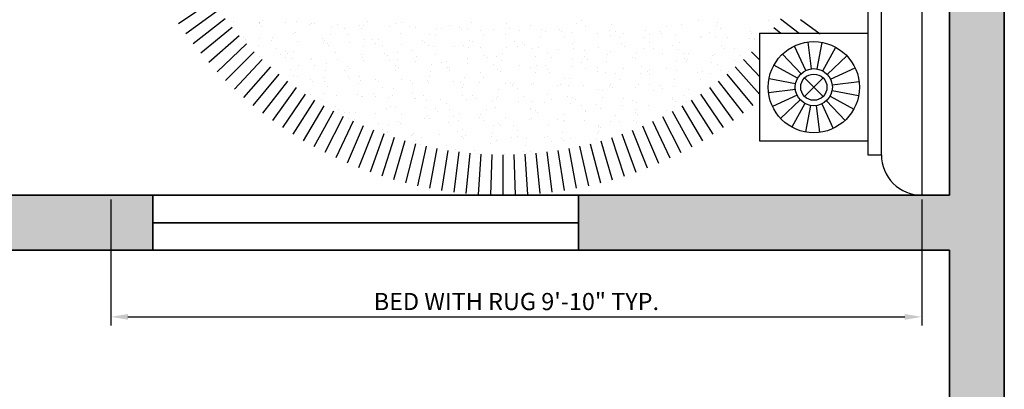
# Model space of a CAD drawing. Units: inches. Extents: x 1566 to 2546, y 1087 to 2705.
# Tile 15 of 27: x 2315 to 2458, y 1189 to 1243. Entities that reach past the tile are written whole.
import ezdxf

# ---------------------------------------------------------------- set-up
doc = ezdxf.new("R2010")
doc.units = ezdxf.units.IN
for name, color, linetype, lineweight in [('A-ANNO-DIMS', 2, 'Continuous', 18), ('A-FURN', 8, 'Continuous', 18), ('A-WALL', 7, 'Continuous', 35), ('A-WALL-PATT', 8, 'Continuous', 13)]:
    doc.layers.add(name, color=color, linetype=linetype, lineweight=lineweight)
for name, color, linetype in [('A-FRN', 11, 'Continuous'), ('A-HT', 15, 'Continuous'), ('L-HT', 1, 'Continuous')]:
    doc.layers.add(name, color=color, linetype=linetype)
doc.styles.get("Standard").update_dxf_attribs({"font": 'arial.ttf'})
doc.dimstyles.new('ISO-25', dxfattribs={"dimtxt": 2.5, "dimasz": 2.5, "dimexe": 1.25, "dimexo": 0.625, "dimtad": 1, "dimtxsty": 'Standard', "dimcen": 2.5, "dimadec": 0, "dimazin": 0, "dimtfac": 1, "dimtmove": 0, "dimatfit": 3, "dimfxl": 1, "dimarcsym": 0})

# ---------------------------------------------------------------- blocks, each defined once
blk = doc.blocks.new('*X21')
at = {"color": 0}
for p, q in [((2.8058, 2.548), (2.8058, 2.548)), ((2.8678, 2.5109), (2.8678, 2.5109)), ((2.8734, 2.5011), (2.8734, 2.5011)), ((2.8889, 2.4975), (2.8889, 2.4975)), ((2.8024, 2.4403), (2.8024, 2.4403)), ((2.8089, 2.4516), (2.8089, 2.4516)), ((2.8091, 2.4488), (2.8091, 2.4488)), ((2.8148, 2.4495), (2.8148, 2.4495)), ((2.824, 2.4411), (2.824, 2.4411)), ((2.8703, 2.4492), (2.8703, 2.4492)), ((2.8963, 2.4526), (2.8963, 2.4526)), ((2.9368, 2.451), (2.9368, 2.451)), ((2.8765, 2.4048), (2.8765, 2.4048)), ((2.8675, 2.4012), (2.8675, 2.4012)), ((2.9082, 2.3857), (2.9082, 2.3857)), ((2.9293, 2.3723), (2.9293, 2.3723)), ((2.8121, 2.3553), (2.8121, 2.3553)), ((2.9173, 2.3556), (2.9173, 2.3556)), ((2.9265, 2.3472), (2.9265, 2.3472)), ((2.94, 2.3547), (2.94, 2.3547)), ((2.983, 2.3346), (2.983, 2.3346)), ((2.8078, 2.3115), (2.8078, 2.3115)), ((2.8485, 2.3169), (2.8485, 2.3169)), ((2.8495, 2.3236), (2.8495, 2.3236)), ((2.8797, 2.3084), (2.8797, 2.3084)), ((2.9164, 2.3258), (2.9164, 2.3258)), ((2.9424, 2.3292), (2.9424, 2.3292)), ((2.97, 2.3073), (2.97, 2.3073)), ((3.0052, 2.3239), (3.0052, 2.3239)), ((3.0106, 2.3101), (3.0106, 2.3101)), ((2.8152, 2.259), (2.8152, 2.259)), ((2.8197, 2.2634), (2.8197, 2.2634)), ((2.9431, 2.2584), (2.9431, 2.2584)), ((2.9486, 2.2605), (2.9486, 2.2605)), ((3.0198, 2.2617), (3.0198, 2.2617)), ((3.0782, 2.2632), (3.0782, 2.2632)), ((2.814, 2.2468), (2.814, 2.2468)), ((2.9697, 2.2471), (2.9697, 2.2471)), ((3.029, 2.2533), (3.029, 2.2533)), ((2.8539, 2.1881), (2.8539, 2.1881)), ((2.8695, 2.2178), (2.8695, 2.2178)), ((2.8787, 2.2094), (2.8787, 2.2094)), ((2.8828, 2.2121), (2.8828, 2.2121)), ((2.8899, 2.1984), (2.8899, 2.1984)), ((2.8946, 2.1935), (2.8946, 2.1935)), ((2.9625, 2.2024), (2.9625, 2.2024)), ((2.9885, 2.2058), (2.9885, 2.2058)), ((3.0137, 2.2138), (3.0137, 2.2138)), ((3.0291, 2.2112), (3.0291, 2.2112)), ((3.0456, 2.1987), (3.0456, 2.1987)), ((3.0725, 2.2134), (3.0725, 2.2134)), ((3.0971, 2.2201), (3.0971, 2.2201)), ((2.8184, 2.1626), (2.8184, 2.1626)), ((2.8279, 2.1847), (2.8279, 2.1847)), ((2.9222, 2.1695), (2.9222, 2.1695)), ((2.9463, 2.162), (2.9463, 2.162)), ((3.0813, 2.1669), (3.0813, 2.1669)), ((3.1223, 2.1678), (3.1223, 2.1678)), ((3.1315, 2.1594), (3.1315, 2.1594)), ((2.8333, 2.135), (2.8333, 2.135)), ((2.8544, 2.1216), (2.8544, 2.1216)), ((2.886, 2.1157), (2.886, 2.1157)), ((2.972, 2.1239), (2.972, 2.1239)), ((2.9812, 2.1155), (2.9812, 2.1155)), ((2.989, 2.1353), (2.989, 2.1353)), ((3.0101, 2.1218), (3.0101, 2.1218)), ((3.0169, 2.1174), (3.0169, 2.1174)), ((3.1447, 2.1356), (3.1447, 2.1356)), ((3.1448, 2.1168), (3.1448, 2.1168)), ((3.1658, 2.1221), (3.1658, 2.1221)), ((2.8216, 2.08), (2.8216, 2.08)), ((3.0086, 2.079), (3.0086, 2.079)), ((3.0346, 2.0825), (3.0346, 2.0825)), ((3.0752, 2.0878), (3.0752, 2.0878)), ((3.1432, 2.0968), (3.1432, 2.0968)), ((3.1692, 2.1002), (3.1692, 2.1002)), ((2.8061, 2.0524), (2.8061, 2.0524)), ((2.8215, 2.0663), (2.8215, 2.0663)), ((2.8309, 2.0716), (2.8309, 2.0716)), ((2.874, 2.0613), (2.874, 2.0613)), ((2.9, 2.0647), (2.9, 2.0647)), ((2.9303, 2.0732), (2.9303, 2.0732)), ((2.9407, 2.0701), (2.9407, 2.0701)), ((2.9494, 2.0657), (2.9494, 2.0657)), ((3.0247, 2.0756), (3.0247, 2.0756)), ((3.0845, 2.0705), (3.0845, 2.0705)), ((3.086, 2.0735), (3.086, 2.0735)), ((2.8737, 2.0098), (2.8737, 2.0098)), ((2.8744, 2.0317), (2.8744, 2.0317)), ((2.8891, 2.0194), (2.8891, 2.0194)), ((3.02, 2.0211), (3.02, 2.0211)), ((3.0294, 2.0101), (3.0294, 2.0101)), ((3.0744, 2.03), (3.0744, 2.03)), ((3.0837, 2.0216), (3.0837, 2.0216)), ((3.1479, 2.0205), (3.1479, 2.0205)), ((3.1851, 2.0104), (3.1851, 2.0104)), ((2.8247, 1.9699), (2.8247, 1.9699)), ((2.8947, 1.9964), (2.8947, 1.9964)), ((2.9241, 1.9861), (2.9241, 1.9861)), ((2.9333, 1.9777), (2.9333, 1.9777)), ((2.9526, 1.9693), (2.9526, 1.9693)), ((3.0505, 1.9966), (3.0505, 1.9966)), ((3.0876, 1.9742), (3.0876, 1.9742)), ((3.1272, 1.9817), (3.1272, 1.9817)), ((3.1893, 1.9734), (3.1893, 1.9734)), ((3.2062, 1.9969), (3.2062, 1.9969)), ((3.2153, 1.9768), (3.2153, 1.9768)), ((3.2185, 1.9759), (3.2185, 1.9759)), ((2.8149, 1.9477), (2.8149, 1.9477)), ((2.9201, 1.9379), (2.9201, 1.9379)), ((2.9461, 1.9414), (2.9461, 1.9414)), ((2.9707, 1.948), (2.9707, 1.948)), ((2.9768, 1.9378), (2.9768, 1.9378)), ((2.9868, 1.9467), (2.9868, 1.9467)), ((3.0547, 1.9556), (3.0547, 1.9556)), ((3.0807, 1.9591), (3.0807, 1.9591)), ((3.1213, 1.9644), (3.1213, 1.9644)), ((3.1264, 1.9483), (3.1264, 1.9483)), ((3.1769, 1.9361), (3.1769, 1.9361)), ((2.8115, 1.9236), (2.8115, 1.9236)), ((2.8265, 1.894), (2.8265, 1.894)), ((2.8522, 1.929), (2.8522, 1.929)), ((2.8923, 1.9231), (2.8923, 1.9231)), ((3.0232, 1.9247), (3.0232, 1.9247)), ((3.1511, 1.9241), (3.1511, 1.9241)), ((3.1861, 1.9277), (3.1861, 1.9277)), ((2.8278, 1.8736), (2.8278, 1.8736)), ((2.914, 1.8846), (2.914, 1.8846)), ((2.9351, 1.8712), (2.9351, 1.8712)), ((2.9557, 1.873), (2.9557, 1.873)), ((3.0266, 1.8922), (3.0266, 1.8922)), ((3.0358, 1.8838), (3.0358, 1.8838)), ((3.0697, 1.8849), (3.0697, 1.8849)), ((3.0908, 1.8779), (3.0908, 1.8779)), ((3.0908, 1.8714), (3.0908, 1.8714)), ((3.2217, 1.8795), (3.2217, 1.8795)), ((3.2255, 1.8852), (3.2255, 1.8852)), ((3.2296, 1.8878), (3.2296, 1.8878)), ((3.2465, 1.8717), (3.2465, 1.8717)), ((2.8553, 1.8225), (2.8553, 1.8225)), ((2.8763, 1.8484), (2.8763, 1.8484)), ((2.8855, 1.8399), (2.8855, 1.8399)), ((2.8954, 1.8267), (2.8954, 1.8267)), ((3.011, 1.8228), (3.011, 1.8228)), ((3.0263, 1.8284), (3.0263, 1.8284)), ((3.0329, 1.8233), (3.0329, 1.8233)), ((3.0793, 1.8439), (3.0793, 1.8439)), ((3.1008, 1.8323), (3.1008, 1.8323)), ((3.1268, 1.8357), (3.1268, 1.8357)), ((3.1542, 1.8278), (3.1542, 1.8278)), ((3.1667, 1.8231), (3.1667, 1.8231)), ((3.1674, 1.841), (3.1674, 1.841)), ((3.2354, 1.85), (3.2354, 1.85)), ((3.2614, 1.8534), (3.2614, 1.8534)), ((2.8316, 1.7968), (2.8316, 1.7968)), ((2.8576, 1.8002), (2.8576, 1.8002)), ((2.8983, 1.8056), (2.8983, 1.8056)), ((2.929, 1.8), (2.929, 1.8)), ((2.9662, 1.8145), (2.9662, 1.8145)), ((2.9922, 1.818), (2.9922, 1.818)), ((3.1291, 1.7983), (3.1291, 1.7983)), ((3.1383, 1.7899), (3.1383, 1.7899)), ((2.831, 1.7773), (2.831, 1.7773)), ((2.9544, 1.7594), (2.9544, 1.7594)), ((2.9589, 1.7766), (2.9589, 1.7766)), ((2.9788, 1.7544), (2.9788, 1.7544)), ((3.0939, 1.7815), (3.0939, 1.7815)), ((3.1101, 1.7597), (3.1101, 1.7597)), ((3.1818, 1.75), (3.1818, 1.75)), ((3.2248, 1.7832), (3.2248, 1.7832)), ((3.2658, 1.7599), (3.2658, 1.7599)), ((2.8198, 1.7457), (2.8198, 1.7457)), ((2.8986, 1.7304), (2.8986, 1.7304)), ((2.9755, 1.7459), (2.9755, 1.7459)), ((2.988, 1.746), (2.988, 1.746)), ((3.0295, 1.7321), (3.0295, 1.7321)), ((3.1312, 1.7462), (3.1312, 1.7462)), ((3.1574, 1.7314), (3.1574, 1.7314)), ((3.1729, 1.7123), (3.1729, 1.7123)), ((3.2135, 1.7176), (3.2135, 1.7176)), ((3.2815, 1.7266), (3.2815, 1.7266)), ((2.8285, 1.7106), (2.8285, 1.7106)), ((2.8341, 1.6809), (2.8341, 1.6809)), ((2.8377, 1.7021), (2.8377, 1.7021)), ((2.8957, 1.6973), (2.8957, 1.6973)), ((2.9037, 1.6769), (2.9037, 1.6769)), ((2.9444, 1.6822), (2.9444, 1.6822)), ((2.962, 1.6803), (2.962, 1.6803)), ((3.0123, 1.6911), (3.0123, 1.6911)), ((3.0315, 1.7061), (3.0315, 1.7061)), ((3.0383, 1.6946), (3.0383, 1.6946)), ((3.0514, 1.6976), (3.0514, 1.6976)), ((3.079, 1.6999), (3.079, 1.6999)), ((3.0971, 1.6852), (3.0971, 1.6852)), ((3.1469, 1.7089), (3.1469, 1.7089)), ((3.2071, 1.6979), (3.2071, 1.6979)), ((3.228, 1.6868), (3.228, 1.6868)), ((3.2316, 1.7044), (3.2316, 1.7044)), ((3.2408, 1.696), (3.2408, 1.696)), ((2.8098, 1.6645), (2.8098, 1.6645)), ((2.8777, 1.6734), (2.8777, 1.6734)), ((2.8812, 1.6623), (2.8812, 1.6623)), ((3.0813, 1.6605), (3.0813, 1.6605)), ((3.0905, 1.6521), (3.0905, 1.6521)), ((3.2843, 1.6561), (3.2843, 1.6561)), ((3.2956, 1.64), (3.2956, 1.64)), ((2.8391, 1.6339), (2.8391, 1.6339)), ((2.8602, 1.6205), (2.8602, 1.6205)), ((2.9017, 1.634), (2.9017, 1.634)), ((2.931, 1.6167), (2.931, 1.6167)), ((2.9402, 1.6082), (2.9402, 1.6082)), ((2.9948, 1.6342), (2.9948, 1.6342)), ((3.0159, 1.6207), (3.0159, 1.6207)), ((3.0326, 1.6357), (3.0326, 1.6357)), ((3.134, 1.6122), (3.134, 1.6122)), ((3.1505, 1.6345), (3.1505, 1.6345)), ((3.1605, 1.6351), (3.1605, 1.6351)), ((3.1716, 1.621), (3.1716, 1.621)), ((2.8373, 1.5846), (2.8373, 1.5846)), ((2.9361, 1.5721), (2.9361, 1.5721)), ((2.9652, 1.584), (2.9652, 1.584)), ((2.9837, 1.5683), (2.9837, 1.5683)), ((3.0584, 1.5678), (3.0584, 1.5678)), ((3.0844, 1.5712), (3.0844, 1.5712)), ((3.0918, 1.5724), (3.0918, 1.5724)), ((3.1002, 1.5888), (3.1002, 1.5888)), ((3.1251, 1.5765), (3.1251, 1.5765)), ((3.1838, 1.5666), (3.1838, 1.5666)), ((3.193, 1.5855), (3.193, 1.5855)), ((3.219, 1.5889), (3.219, 1.5889)), ((3.2311, 1.5905), (3.2311, 1.5905)), ((3.2475, 1.5727), (3.2475, 1.5727)), ((3.2596, 1.5943), (3.2596, 1.5943)), ((2.8152, 1.5357), (2.8152, 1.5357)), ((2.8559, 1.5411), (2.8559, 1.5411)), ((2.9049, 1.5377), (2.9049, 1.5377)), ((2.9238, 1.55), (2.9238, 1.55)), ((2.9498, 1.5535), (2.9498, 1.5535)), ((2.9905, 1.5588), (2.9905, 1.5588)), ((3.0358, 1.5394), (3.0358, 1.5394)), ((3.1637, 1.5388), (3.1637, 1.5388)), ((3.193, 1.5582), (3.193, 1.5582)), ((3.2987, 1.5436), (3.2987, 1.5436)), ((2.8334, 1.5245), (2.8334, 1.5245)), ((2.8795, 1.5087), (2.8795, 1.5087)), ((2.9006, 1.4953), (2.9006, 1.4953)), ((3.0334, 1.5227), (3.0334, 1.5227)), ((3.0352, 1.509), (3.0352, 1.509)), ((3.0427, 1.5143), (3.0427, 1.5143)), ((3.0563, 1.4955), (3.0563, 1.4955)), ((3.1909, 1.5093), (3.1909, 1.5093)), ((3.212, 1.4958), (3.212, 1.4958)), ((3.2343, 1.4942), (3.2343, 1.4942)), ((3.2365, 1.5183), (3.2365, 1.5183)), ((2.8404, 1.4882), (2.8404, 1.4882)), ((2.8831, 1.4789), (2.8831, 1.4789)), ((2.8924, 1.4704), (2.8924, 1.4704)), ((2.9683, 1.4876), (2.9683, 1.4876)), ((3.0862, 1.4744), (3.0862, 1.4744)), ((3.1034, 1.4925), (3.1034, 1.4925)), ((3.2391, 1.4621), (3.2391, 1.4621)), ((3.2651, 1.4655), (3.2651, 1.4655)), ((3.2862, 1.4727), (3.2862, 1.4727)), ((3.2954, 1.4643), (3.2954, 1.4643)), ((2.8208, 1.4466), (2.8208, 1.4466)), ((2.908, 1.4414), (2.908, 1.4414)), ((2.9359, 1.4306), (2.9359, 1.4306)), ((2.9699, 1.4267), (2.9699, 1.4267)), ((2.9765, 1.4469), (2.9765, 1.4469)), ((2.9959, 1.4301), (2.9959, 1.4301)), ((3.0366, 1.4354), (3.0366, 1.4354)), ((3.0389, 1.443), (3.0389, 1.443)), ((3.1045, 1.4444), (3.1045, 1.4444)), ((3.1305, 1.4478), (3.1305, 1.4478)), ((3.1322, 1.4472), (3.1322, 1.4472)), ((3.1359, 1.4288), (3.1359, 1.4288)), ((3.1451, 1.4204), (3.1451, 1.4204)), ((3.1668, 1.4424), (3.1668, 1.4424)), ((3.1712, 1.4532), (3.1712, 1.4532)), ((3.2879, 1.4475), (3.2879, 1.4475)), ((2.8353, 1.4089), (2.8353, 1.4089)), ((2.8436, 1.3919), (2.8436, 1.3919)), ((2.8613, 1.4124), (2.8613, 1.4124)), ((2.902, 1.4177), (2.902, 1.4177)), ((2.9715, 1.3913), (2.9715, 1.3913)), ((2.9856, 1.385), (2.9856, 1.385)), ((3.0756, 1.3838), (3.0756, 1.3838)), ((3.1065, 1.3961), (3.1065, 1.3961)), ((3.2313, 1.384), (3.2313, 1.384)), ((3.2374, 1.3978), (3.2374, 1.3978)), ((2.9199, 1.3835), (2.9199, 1.3835)), ((2.9409, 1.37), (2.9409, 1.37)), ((2.9948, 1.3765), (2.9948, 1.3765)), ((3.0967, 1.3703), (3.0967, 1.3703)), ((3.1886, 1.3805), (3.1886, 1.3805)), ((3.2524, 1.3706), (3.2524, 1.3706)), ((2.8353, 1.3411), (2.8353, 1.3411)), ((2.8445, 1.3326), (2.8445, 1.3326)), ((2.8611, 1.3214), (2.8611, 1.3214)), ((2.9112, 1.345), (2.9112, 1.345)), ((3.0169, 1.3217), (3.0169, 1.3217)), ((3.0383, 1.3367), (3.0383, 1.3367)), ((3.0421, 1.3467), (3.0421, 1.3467)), ((3.0827, 1.312), (3.0827, 1.312)), ((3.1506, 1.321), (3.1506, 1.321)), ((3.17, 1.3461), (3.17, 1.3461)), ((3.1726, 1.322), (3.1726, 1.322)), ((3.1766, 1.3244), (3.1766, 1.3244)), ((3.2173, 1.3298), (3.2173, 1.3298)), ((3.2384, 1.3349), (3.2384, 1.3349)), ((3.2476, 1.3265), (3.2476, 1.3265)), ((2.8135, 1.2766), (2.8135, 1.2766)), ((2.8467, 1.2956), (2.8467, 1.2956)), ((2.8814, 1.2855), (2.8814, 1.2855)), ((2.888, 1.2928), (2.888, 1.2928)), ((2.9074, 1.289), (2.9074, 1.289)), ((2.9481, 1.2943), (2.9481, 1.2943)), ((2.9746, 1.2949), (2.9746, 1.2949)), ((3.016, 1.3033), (3.016, 1.3033)), ((3.042, 1.3067), (3.042, 1.3067)), ((3.0881, 1.291), (3.0881, 1.291)), ((3.0973, 1.2826), (3.0973, 1.2826)), ((3.1097, 1.2998), (3.1097, 1.2998)), ((3.2406, 1.3015), (3.2406, 1.3015)), ((2.8045, 1.258), (2.8045, 1.258)), ((2.8256, 1.2446), (2.8256, 1.2446)), ((2.9143, 1.2487), (2.9143, 1.2487)), ((2.9378, 1.2472), (2.9378, 1.2472)), ((2.947, 1.2387), (2.947, 1.2387)), ((2.9602, 1.2583), (2.9602, 1.2583)), ((2.9813, 1.2448), (2.9813, 1.2448)), ((3.0452, 1.2503), (3.0452, 1.2503)), ((3.1159, 1.2586), (3.1159, 1.2586)), ((3.137, 1.2451), (3.137, 1.2451)), ((3.1408, 1.2427), (3.1408, 1.2427)), ((3.1731, 1.2497), (3.1731, 1.2497)), ((3.1128, 1.2035), (3.1128, 1.2035)), ((3.2437, 1.2051), (3.2437, 1.2051)), ((2.8499, 1.1992), (2.8499, 1.1992)), ((2.9015, 1.1962), (2.9015, 1.1962)), ((2.9535, 1.1656), (2.9535, 1.1656)), ((2.9778, 1.1986), (2.9778, 1.1986)), ((2.9905, 1.1989), (2.9905, 1.1989)), ((2.9942, 1.1709), (2.9942, 1.1709)), ((3.0572, 1.1965), (3.0572, 1.1965)), ((3.0621, 1.1799), (3.0621, 1.1799)), ((3.0881, 1.1833), (3.0881, 1.1833)), ((3.1288, 1.1887), (3.1288, 1.1887)), ((3.1906, 1.1971), (3.1906, 1.1971)), ((3.1967, 1.1976), (3.1967, 1.1976)), ((3.1998, 1.1887), (3.1998, 1.1887)), ((3.2129, 1.1968), (3.2129, 1.1968)), ((3.2227, 1.201), (3.2227, 1.201)), ((2.8189, 1.1479), (2.8189, 1.1479)), ((2.8402, 1.155), (2.8402, 1.155)), ((2.8449, 1.1328), (2.8449, 1.1328)), ((2.8596, 1.1532), (2.8596, 1.1532)), ((2.9175, 1.1523), (2.9175, 1.1523)), ((2.9275, 1.1622), (2.9275, 1.1622)), ((3.0006, 1.1331), (3.0006, 1.1331)), ((3.0403, 1.1533), (3.0403, 1.1533)), ((3.0484, 1.154), (3.0484, 1.154)), ((3.0495, 1.1448), (3.0495, 1.1448)), ((3.1563, 1.1334), (3.1563, 1.1334)), ((3.1763, 1.1534), (3.1763, 1.1534)), ((2.853, 1.1029), (2.853, 1.1029)), ((2.866, 1.1194), (2.866, 1.1194)), ((2.89, 1.1094), (2.89, 1.1094)), ((2.8992, 1.1009), (2.8992, 1.1009)), ((2.9809, 1.1023), (2.9809, 1.1023)), ((3.0217, 1.1196), (3.0217, 1.1196)), ((3.093, 1.105), (3.093, 1.105)), ((3.116, 1.1071), (3.116, 1.1071)), ((3.1774, 1.1199), (3.1774, 1.1199)), ((2.9419, 1.071), (2.9419, 1.071)), ((2.9427, 1.0611), (2.9427, 1.0611)), ((3.0515, 1.0577), (3.0515, 1.0577)), ((3.0976, 1.0713), (3.0976, 1.0713)), ((3.1082, 1.0565), (3.1082, 1.0565)), ((3.1342, 1.0599), (3.1342, 1.0599)), ((3.1428, 1.0594), (3.1428, 1.0594)), ((3.1749, 1.0653), (3.1749, 1.0653)), ((3.1794, 1.057), (3.1794, 1.057)), ((2.839, 1.0211), (2.839, 1.0211)), ((2.865, 1.0245), (2.865, 1.0245)), ((2.9057, 1.0298), (2.9057, 1.0298)), ((2.9206, 1.056), (2.9206, 1.056)), ((2.9736, 1.0388), (2.9736, 1.0388)), ((2.9996, 1.0422), (2.9996, 1.0422)), ((3.0403, 1.0475), (3.0403, 1.0475)), ((3.152, 1.0509), (3.152, 1.0509)), ((2.8562, 1.0065), (2.8562, 1.0065)), ((2.8853, 1.0076), (2.8853, 1.0076)), ((2.9064, 0.9942), (2.9064, 0.9942)), ((2.9841, 1.0059), (2.9841, 1.0059)), ((2.9925, 1.0155), (2.9925, 1.0155)), ((3.0017, 1.007), (3.0017, 1.007)), ((3.041, 1.0079), (3.041, 1.0079)), ((3.0621, 0.9944), (3.0621, 0.9944)), ((3.1191, 1.0108), (3.1191, 1.0108)), ((2.8421, 0.9716), (2.8421, 0.9716)), ((2.8514, 0.9631), (2.8514, 0.9631)), ((2.9238, 0.9597), (2.9238, 0.9597)), ((3.0452, 0.9672), (3.0452, 0.9672)), ((3.0547, 0.9613), (3.0547, 0.9613)), ((2.8266, 0.9455), (2.8266, 0.9455)), ((2.8949, 0.9233), (2.8949, 0.9233)), ((2.9823, 0.9458), (2.9823, 0.9458)), ((3.0197, 0.9154), (3.0197, 0.9154)), ((3.0457, 0.9188), (3.0457, 0.9188)), ((3.0864, 0.9242), (3.0864, 0.9242)), ((3.0949, 0.9216), (3.0949, 0.9216)), ((3.1041, 0.9131), (3.1041, 0.9131)), ((3.1223, 0.9144), (3.1223, 0.9144)), ((3.138, 0.9461), (3.138, 0.9461)), ((2.8172, 0.8887), (2.8172, 0.8887)), ((2.8593, 0.9102), (2.8593, 0.9102)), ((2.8851, 0.8977), (2.8851, 0.8977)), ((2.9111, 0.9011), (2.9111, 0.9011)), ((2.9257, 0.8824), (2.9257, 0.8824)), ((2.9446, 0.8777), (2.9446, 0.8777)), ((2.9518, 0.9064), (2.9518, 0.9064)), ((2.9872, 0.9096), (2.9872, 0.9096)), ((3.0814, 0.8827), (3.0814, 0.8827)), ((2.9269, 0.8633), (2.9269, 0.8633)), ((2.9468, 0.8689), (2.9468, 0.8689)), ((2.9538, 0.8692), (2.9538, 0.8692)), ((3.0578, 0.865), (3.0578, 0.865)), ((3.1025, 0.8692), (3.1025, 0.8692)), ((2.8035, 0.8253), (2.8035, 0.8253)), ((2.8625, 0.8138), (2.8625, 0.8138)), ((2.867, 0.8203), (2.867, 0.8203)), ((2.9904, 0.8132), (2.9904, 0.8132)), ((2.9973, 0.8294), (2.9973, 0.8294)), ((3.0227, 0.8206), (3.0227, 0.8206)), ((2.847, 0.7855), (2.847, 0.7855)), ((2.8633, 0.7653), (2.8633, 0.7653)), ((2.9301, 0.767), (2.9301, 0.767)), ((2.9312, 0.7743), (2.9312, 0.7743)), ((2.9572, 0.7777), (2.9572, 0.7777)), ((2.9979, 0.7831), (2.9979, 0.7831)), ((3.0471, 0.7838), (3.0471, 0.7838)), ((2.8104, 0.7569), (2.8104, 0.7569)), ((2.8227, 0.76), (2.8227, 0.76)), ((2.8314, 0.7435), (2.8314, 0.7435)), ((2.8968, 0.7399), (2.8968, 0.7399)), ((2.906, 0.7314), (2.906, 0.7314)), ((2.9661, 0.7572), (2.9661, 0.7572)), ((2.9871, 0.7437), (2.9871, 0.7437)), ((2.8656, 0.7175), (2.8656, 0.7175)), ((2.9073, 0.6951), (2.9073, 0.6951)), ((2.9935, 0.7169), (2.9935, 0.7169)), ((2.9332, 0.6706), (2.9332, 0.6706)), ((2.9495, 0.6916), (2.9495, 0.6916)), ((2.8427, 0.6332), (2.8427, 0.6332)), ((2.8507, 0.6317), (2.8507, 0.6317)), ((2.8688, 0.6366), (2.8688, 0.6366)), ((2.8688, 0.6212), (2.8688, 0.6212)), ((2.9094, 0.6419), (2.9094, 0.6419)), ((2.849, 0.6021), (2.849, 0.6021)), ((2.8718, 0.6183), (2.8718, 0.6183)), ((2.8013, 0.5694), (2.8013, 0.5694))]:
    blk.add_line(p, q, dxfattribs=at)
blk = doc.blocks.new('A$C6796526C')
at = {"layer": 'A-FRN'}
for p, q in [((0, 3), (2.9, 3)), ((2.75, 2.85), (0.15, 2.85)), ((2.75, 2.8), (2.75, 2.85)), ((0.15, 2.8), (2.75, 2.8)), ((2.3, 2.4), (2.3, 2.8)), ((2.7, 2.8), (2.7, 2.4)), ((2.7, 2.4), (2.3, 2.4))]:
    blk.add_line(p, q, dxfattribs=at)
for radius in [0.1686, 0.0686]:
    blk.add_circle((2.5, 2.6), radius, dxfattribs=at)
blk.add_arc((2.75, 3), 0.15, 270, 0, dxfattribs=at)
at = {"layer": 'A-HT'}
for p, q in [((2.25, 2.5511), (2.3023, 2.6231)), ((2.2468, 2.4772), (2.3, 2.5458)), ((2.2787, 2.4517), (2.3, 2.4775)), ((2.3692, 2.3692), (2.4, 2.4)), ((2.3977, 2.3399), (2.4616, 2.4)), ((2.4251, 2.3097), (2.5276, 2.4)), ((2.4517, 2.2787), (2.5672, 2.3743)), ((2.4772, 2.2468), (2.5957, 2.3387)), ((2.5017, 2.2141), (2.6231, 2.3023)), ((2.5252, 2.1807), (2.6493, 2.265)), ((2.5476, 2.1466), (2.6743, 2.2269)), ((2.569, 2.1118), (2.6981, 2.1881)), ((2.5892, 2.0763), (2.7206, 2.1485)), ((2.6083, 2.0402), (2.742, 2.1083)), ((2.6263, 2.0035), (2.762, 2.0674)), ((2.6431, 1.9663), (2.7807, 2.0259)), ((2.6587, 1.9286), (2.7982, 1.9838)), ((2.6731, 1.8904), (2.8143, 1.9412)), ((2.6864, 1.8517), (2.829, 1.8981)), ((2.6984, 1.8127), (2.8424, 1.8545)), ((2.7092, 1.7733), (2.8544, 1.8106)), ((2.7187, 1.7336), (2.8651, 1.7663)), ((2.727, 1.6936), (2.8743, 1.7217)), ((2.734, 1.6534), (2.8821, 1.6768)), ((2.7397, 1.6129), (2.8886, 1.6317)), ((2.7442, 1.5723), (2.8936, 1.5865)), ((2.7474, 1.5316), (2.8971, 1.541)), ((2.7494, 1.4908), (2.8993, 1.4955)), ((2.75, 1.45), (2.9, 1.45)), ((2.7494, 1.4092), (2.8993, 1.4045)), ((2.7474, 1.3684), (2.8971, 1.359)), ((2.7442, 1.3277), (2.8936, 1.3135)), ((2.7397, 1.2871), (2.8886, 1.2683)), ((2.734, 1.2466), (2.8821, 1.2232)), ((2.727, 1.2064), (2.8743, 1.1783)), ((2.7187, 1.1664), (2.8651, 1.1337)), ((2.7092, 1.1267), (2.8544, 1.0894)), ((2.6984, 1.0873), (2.8424, 1.0455)), ((2.6864, 1.0483), (2.829, 1.0019)), ((2.6731, 1.0096), (2.8143, 0.9588)), ((2.6587, 0.9714), (2.7982, 0.9162)), ((2.6431, 0.9337), (2.7807, 0.8741)), ((2.6263, 0.8965), (2.762, 0.8326)), ((2.6083, 0.8598), (2.742, 0.7917)), ((2.5892, 0.8237), (2.7206, 0.7515)), ((2.569, 0.7882), (2.6981, 0.7119)), ((2.5476, 0.7534), (2.6743, 0.6731)), ((2.5252, 0.7193), (2.6493, 0.635)), ((2.5017, 0.6859), (2.6231, 0.5977)), ((2.4517, 0.6213), (2.5672, 0.5257)), ((2.4772, 0.6532), (2.5957, 0.5613)), ((2.4251, 0.5903), (2.5377, 0.4911)), ((2.3977, 0.5601), (2.507, 0.4574)), ((2.3692, 0.5308), (2.4753, 0.4247)), ((2.3097, 0.4749), (2.4089, 0.3623)), ((2.3399, 0.5023), (2.4426, 0.393)), ((2.2787, 0.4483), (2.3743, 0.3328)), ((2.2474, 0.423), (2.3394, 0.3045)), ((2.1814, 0.375), (2.2657, 0.251)), ((2.2148, 0.3985), (2.303, 0.2772))]:
    blk.add_line(p, q, dxfattribs=at)
at = {"layer": 'L-HT'}
for p, q in [((2.4707, 2.662), (2.428, 2.7524)), ((2.4913, 2.668), (2.4786, 2.7672)), ((2.5127, 2.6674), (2.5313, 2.7656)), ((2.5329, 2.6601), (2.581, 2.7478)), ((2.453, 2.6499), (2.3844, 2.7227)), ((2.5499, 2.647), (2.6227, 2.7156)), ((2.4399, 2.6329), (2.3522, 2.681)), ((2.562, 2.6293), (2.6524, 2.672)), ((2.4326, 2.6127), (2.3344, 2.6313)), ((2.4657, 2.5657), (2.5343, 2.6343)), ((2.5343, 2.5657), (2.4657, 2.6343)), ((2.432, 2.5913), (2.3328, 2.5786)), ((2.5674, 2.5873), (2.6656, 2.5687)), ((2.568, 2.6087), (2.6672, 2.6214)), ((2.438, 2.5707), (2.3476, 2.528)), ((2.4501, 2.553), (2.3773, 2.4844)), ((2.547, 2.5501), (2.6156, 2.4773)), ((2.5601, 2.5671), (2.6478, 2.519)), ((2.4671, 2.5399), (2.419, 2.4522)), ((2.4873, 2.5326), (2.4687, 2.4344)), ((2.5087, 2.532), (2.5214, 2.4328)), ((2.5293, 2.538), (2.572, 2.4476))]:
    blk.add_line(p, q, dxfattribs=at)
blk.add_circle((2.5, 2.6), 0.0486, dxfattribs=at)
at = {"layer": 'A-HT', "extrusion": (0, 0, -1), "zscale": -1, "rotation": 180}
blk.add_blockref('*X21', (0.55, 3), dxfattribs=at)
blk = doc.blocks.new('*D47')
at = {"layer": 'A-ANNO-DIMS', "color": 0, "lineweight": -2, "transparency": 16777216}
for p, q in [((2328.19, 1216.81), (2328.19, 1198.47)), ((2446.3, 1216.81), (2446.3, 1198.47)), ((2330.69, 1199.72), (2443.8, 1199.72))]:
    blk.add_line(p, q, dxfattribs=at)
at = {"layer": 'A-ANNO-DIMS', "color": 0, "transparency": 16777216}
for points in [[(2330.69, 1200.13), (2330.69, 1199.3), (2328.19, 1199.72)], [(2443.8, 1200.13), (2443.8, 1199.3), (2446.3, 1199.72)]]:
    blk.add_solid(points, dxfattribs=at)
at = {"layer": 'Defpoints', "color": 0, "transparency": 16777216}
for p in [(2328.19, 1217.43), (2446.3, 1217.43), (2446.3, 1199.72)]:
    blk.add_point(p, dxfattribs=at)
at = {"layer": 'A-ANNO-DIMS', "color": 0, "transparency": 16777216, "insert": (2387.25, 1201.63), "char_height": 2.5, "attachment_point": 5}
blk.add_mtext('BED WITH RUG 9\'-10" TYP.', dxfattribs=at)
blk = doc.blocks.new('*D48')
at = {"layer": 'A-ANNO-DIMS', "color": 0, "lineweight": -2, "transparency": 16777216}
for p, q in [((2327.57, 1331.61), (2309.22, 1331.61)), ((2310.47, 1329.11), (2310.47, 1219.93)), ((2327.57, 1217.43), (2309.22, 1217.43))]:
    blk.add_line(p, q, dxfattribs=at)
at = {"layer": 'A-ANNO-DIMS', "color": 0, "transparency": 16777216}
for points in [[(2310.06, 1329.11), (2310.89, 1329.11), (2310.47, 1331.61)], [(2310.06, 1219.93), (2310.89, 1219.93), (2310.47, 1217.43)]]:
    blk.add_solid(points, dxfattribs=at)
at = {"layer": 'Defpoints', "color": 0, "transparency": 16777216}
for p in [(2328.19, 1331.61), (2310.47, 1217.43), (2328.19, 1217.43)]:
    blk.add_point(p, dxfattribs=at)
at = {"layer": 'A-ANNO-DIMS', "color": 0, "transparency": 16777216, "insert": (2308.57, 1274.52), "char_height": 2.5, "attachment_point": 5, "rotation": 90}
blk.add_mtext('9\'-6" TYP.', dxfattribs=at)

msp = doc.modelspace()

# ---------------------------------------------------------------- hatches: boundary and pattern name
at = {"layer": 'A-WALL-PATT'}
h = msp.add_hatch(color=256, dxfattribs=at)
h.dxf.hatch_style = 1
h.paths.add_polyline_path([(2106.29, 1385.43), (2228.29, 1385.43), (2228.29, 1391.43), (2224.29, 1391.43), (2224.29, 1389.43), (2106.29, 1389.43), (2106.29, 1402.93), (2098.29, 1402.93), (2098.29, 1343.43), (2106.29, 1343.43), (2106.29, 1347.74)], flags=17)
h.paths.add_polyline_path([(2106.29, 1259.43), (2098.29, 1259.43), (2098.29, 1209.43), (2155.29, 1209.43), (2155.29, 1217.43), (2143.41, 1217.43), (2106.29, 1217.43)], flags=17)
h.paths.add_polyline_path([(2334.29, 1217.43), (2280.29, 1217.43), (2280.29, 1389.43), (2284.29, 1389.43), (2284.29, 1391.43), (2284.29, 1393.43), (2276.29, 1393.43), (2276.29, 1217.43), (2227.29, 1217.43), (2227.29, 1209.43), (2334.29, 1209.43)], flags=17)
h.paths.add_polyline_path([(2106.29, 1486.43), (2098.29, 1486.43), (2098.29, 1460.88), (2099.11, 1461.64), (2100.44, 1462.65), (2101.57, 1463.26), (2099.97, 1460.62), (2098.29, 1458.1), (2098.29, 1456.93), (2100.35, 1456.93), (2100.77, 1457.12), (2103.56, 1457.95), (2106.29, 1458.4), (2106.29, 1470.43), (2224.29, 1470.43), (2224.29, 1427.43), (2228.29, 1427.43), (2228.29, 1474.43), (2192.29, 1474.43), (2192.29, 1476.43), (2188.29, 1476.43), (2188.29, 1474.43), (2106.29, 1474.43)], flags=17)
h.paths.add_polyline_path([(2106.29, 1585.43), (2192.29, 1585.43), (2192.29, 1589.43), (2098.29, 1589.43), (2098.29, 1573.93), (2106.29, 1573.93)], flags=17)
h.paths.add_polyline_path([(2228.29, 1585.43), (2232.29, 1585.43), (2232.29, 1589.43), (2224.29, 1589.43), (2222.29, 1589.43), (2222.29, 1585.43), (2224.29, 1585.43), (2224.29, 1532.43), (2106.29, 1532.43), (2106.29, 1543.93), (2098.29, 1543.93), (2098.29, 1516.43), (2106.29, 1516.43), (2106.29, 1528.43), (2188.29, 1528.43), (2188.29, 1506.43), (2192.29, 1506.43), (2192.29, 1528.43), (2224.29, 1528.43), (2224.29, 1506.43), (2228.29, 1506.43)], flags=17)
h.paths.add_polyline_path([(2106.29, 1680.43), (2098.29, 1680.43), (2098.29, 1625.43), (2106.29, 1625.43)], flags=17)
h.paths.add_polyline_path([(2458.29, 1784.43), (2098.29, 1784.43), (2098.29, 1776.43), (2276.29, 1776.43), (2276.29, 1589.43), (2268.29, 1589.43), (2268.29, 1585.43), (2280.29, 1585.43), (2280.29, 1652.43), (2284.29, 1652.43), (2284.29, 1656.43), (2280.29, 1656.43), (2280.29, 1776.43), (2398.29, 1776.43), (2398.29, 1746.43), (2402.29, 1746.43), (2402.29, 1776.43), (2450.29, 1776.43), (2450.29, 1532.43), (2375.49, 1532.43), (2328.29, 1532.43), (2328.29, 1612.43), (2324.29, 1612.43), (2324.29, 1528.43), (2450.29, 1528.43), (2450.29, 1447.43), (2291.29, 1447.43), (2291.29, 1443.43), (2324.29, 1443.43), (2324.29, 1393.43), (2320.29, 1393.43), (2320.29, 1389.43), (2330.29, 1389.43), (2330.29, 1393.43), (2328.29, 1393.43), (2328.29, 1443.43), (2412.29, 1443.43), (2412.29, 1433.43), (2416.29, 1433.43), (2416.29, 1443.43), (2450.29, 1443.43), (2450.29, 1393.43), (2416.29, 1393.43), (2416.29, 1403.43), (2412.29, 1403.43), (2412.29, 1393.43), (2360.29, 1393.43), (2360.29, 1389.43), (2450.29, 1389.43), (2450.29, 1217.43), (2396.29, 1217.43), (2396.29, 1209.43), (2450.29, 1209.43), (2450.29, 1136.43), (2458.29, 1136.43)])

# ---------------------------------------------------------------- linework, layer by layer
at = {"layer": 'A-WALL'}
for p, q in [((2458.29, 1784.43), (2458.29, 1136.43)), ((2450.29, 1389.43), (2450.29, 1217.43)), ((2280.29, 1217.43), (2450.29, 1217.43)), ((2334.29, 1217.43), (2334.29, 1209.43)), ((2396.29, 1217.43), (2396.29, 1209.43)), ((2334.29, 1213.43), (2396.29, 1213.43)), ((2098.29, 1209.43), (2450.29, 1209.43)), ((2450.29, 1209.43), (2450.29, 1136.43))]:
    msp.add_line(p, q, dxfattribs=at)

# ---------------------------------------------------------------- block references
at = {"layer": 'A-FURN', "xscale": 39.3701, "yscale": 39.3701, "zscale": 39.3701, "rotation": 270}
msp.add_blockref('A$C6796526C', (2328.19, 1331.61), dxfattribs=at)

# ---------------------------------------------------------------- dimensions: what is measured, and where the dimension line sits
at = {"layer": 'A-ANNO-DIMS'}
dim = msp.add_linear_dim(base=(2310.47, 1217.43), p1=(2328.19, 1331.61), p2=(2328.19, 1217.43), angle=270, text='<> TYP.', dimstyle='ISO-25', override={"dimdec": 1, "dimrnd": 0, "dimzin": 1, "dimlunit": 4, "dimfrac": 2}, dxfattribs=at)
dim.commit()
dim.dimension.update_dxf_attribs({"geometry": '*D48', "text_midpoint": (2308.57, 1274.52)})
dim = msp.add_linear_dim(base=(2446.3, 1199.72), p1=(2328.19, 1217.43), p2=(2446.3, 1217.43), text='BED WITH RUG <> TYP.', dimstyle='ISO-25', override={"dimdec": 1, "dimrnd": 0, "dimzin": 1, "dimlunit": 4, "dimfrac": 2}, dxfattribs=at)
dim.commit()
dim.dimension.update_dxf_attribs({"geometry": '*D47', "text_midpoint": (2387.25, 1201.63)})

doc.saveas('drawing.dxf')
